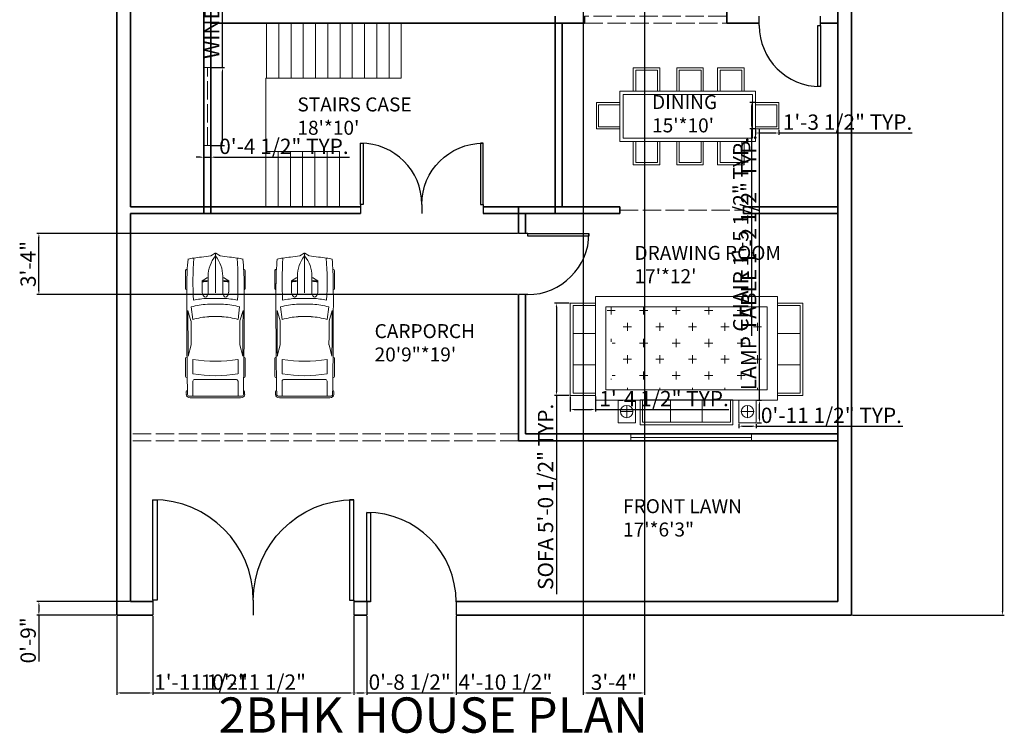
# Model space of a CAD drawing. Units: inches. Extents: x 745 to 1453, y 1850 to 2879.
# Tile 1 of 2: x 745 to 1389, y 1850 to 2316. Entities that reach past the tile are written whole.
import ezdxf

# ---------------------------------------------------------------- set-up
doc = ezdxf.new("R2010")
doc.units = ezdxf.units.IN
doc.linetypes.add('ACAD_ISO02W100', pattern=[15, 12, -3])
for name, color, linetype, lineweight in [('A-ANNO-DIMS', 210, 'Continuous', 18), ('A-ANNO-TEXT', 210, 'Continuous', 25), ('A-AREA-IDEN', 210, 'Continuous', 18), ('A-FLOR-STRS', 92, 'Continuous', 18), ('A-FURN-PATT', 140, 'Continuous', 13), ('A-GLAZ', 4, 'Continuous', 18), ('A-GLAZ-HIGH', 4, 'ACAD_ISO02W100', 18), ('A-WALL-OVHD', 92, 'ACAD_ISO02W100', 18), ('CAR', 10, 'Continuous', 13), ('DOOR', 50, 'Continuous', 25), ('FUR', 140, 'Continuous', 18), ('WALL', 92, 'Continuous', 35)]:
    doc.layers.add(name, color=color, linetype=linetype, lineweight=lineweight)
doc.styles.get("Standard").update_dxf_attribs({"font": 'arial.ttf'})
doc.dimstyles.new('ISO-25', dxfattribs={"dimtxt": 10, "dimasz": 2.5, "dimexe": 1.25, "dimexo": 0.625, "dimtad": 1, "dimdec": 0, "dimlunit": 4, "dimtxsty": 'Standard', "dimcen": 2.5, "dimadec": 0, "dimazin": 0, "dimtfac": 1, "dimtdec": 0, "dimtmove": 0, "dimatfit": 3, "dimfxl": 1, "dimarcsym": 0})

# ---------------------------------------------------------------- blocks, each defined once
blk = doc.blocks.new('*U2')
for p, q in [((0, 0), (0, -6)), ((40, 0), (40, -6))]:
    blk.add_line(p, q)
blk.add_lwpolyline([(0, 0), (0, 40), (1.75, 40), (1.75, 0)], close=True)
blk.add_arc((0, 0), 40, 0, 90)
blk = doc.blocks.new('*U6')
for p, q in [((46.6, 38.9), (22.4, 38.9)), ((136.7, 38.9), (160.9, 38.9)), ((21.1, 37.4), (21.1, 36.8)), ((47.8, 37.4), (47.8, 37.4)), ((70, 31.5), (86.4, 29.4)), ((88, 31.9), (74.8, 35.9)), ((134.3, 35.6), (119.3, 31.8)), ((135.5, 37.1), (135.5, 37.4)), ((138.4, 29.4), (157.2, 29.4)), ((162.1, 37.4), (162.1, 36.8)), ((164.5, 26.4), (164.5, -26.4)), ((186.5, 29.4), (167, 29.4)), ((186.5, -33.5), (186.5, 33.5)), ((188.4, -32.8), (188.4, 32.8)), ((32.3, 11.6), (36.1, 17.2)), ((36.1, 17.2), (50.9, 17.2)), ((3.3, 6.1), (0.1, 0.4)), ((29.8, 9.5), (51.7, 9.5)), ((32.1, 9.5), (32.1, 11.2)), ((58.9, -10.8), (58.9, 10.8)), ((66.6, -10.5), (66.6, 10.5)), ((82.7, 8.5), (82.7, -8.5)), ((186.5, -10.5), (186.5, 10.5)), ((0, 0), (51.7, 0)), ((0.1, -0.4), (3.3, -6.1)), ((29.8, -9.5), (51.7, -9.5)), ((32.1, -9.5), (32.1, -11.2)), ((32.3, -11.6), (36.1, -17.2)), ((36.1, -17.2), (50.9, -17.2)), ((21.1, -37.4), (21.1, -36.8)), ((47.8, -37.4), (47.8, -37.4)), ((86.4, -29.4), (70, -31.5)), ((88, -31.9), (74.8, -35.9)), ((134.3, -35.6), (119.3, -31.8)), ((135.5, -37.1), (135.5, -37.4)), ((157.2, -29.4), (138.4, -29.4)), ((162.1, -37.4), (162.1, -36.8)), ((167, -29.4), (186.5, -29.4)), ((46.6, -38.9), (22.4, -38.9)), ((136.7, -38.9), (160.9, -38.9))]:
    blk.add_line(p, q)
for centre, major_axis, ratio, start_param, end_param in [((22.4, 37.4), (0, -1.48), 0.842304, 3.141593, 4.712389), ((46.6, 37.4), (0, 1.48), 0.842304, -1.570796, 0), ((136.7, 37.4), (0, -1.48), 0.842304, 3.141593, 4.712389), ((160.9, 37.4), (0, 1.48), 0.842304, -1.570796, 0), ((259.2, -27.5), (0, -305.3), 0.842304, 4.528606, 4.561838), ((266, -27.5), (0, 313.3), 0.842304, 1.367076, 1.39176), ((37.5, -594), (0, -623.3), 0.842304, 3.096046, 3.200911), ((41.2, -490.9), (0, 528.2), 0.842304, 0.00281, 0.075598), ((64.5, -10555.6), (0, 10593), 0.842304, -0.013397, 0.002797), ((134.4, 5.4), (0, -89.8), 0.842304, 4.449482, 4.652344), ((135.3, 5.4), (0, 81.8), 0.842304, 1.245306, 1.50788), ((64.5, -10555.6), (0, -10591.5), 0.842304, 3.133765, 3.140441), ((149.6, 2.8), (0, -79.6), 0.842304, 4.372215, 4.640744), ((95.8, -3666.4), (0, -3698.2), 0.842304, 3.134049, 3.144098), ((17.1, 0), (0, 147), 0.842304, 4.511394, 4.913384), ((35.9, 0), (0, 147), 0.842304, 4.511394, 4.913384), ((167, 26.4), (0, 2.96), 0.842304, 0, 1.570796), ((180.6, 35.8), (0, 2.22), 0.842304, -0.013017, 1.249894), ((64.5, -10556.4), (0, 10595.3), 0.842304, -0.013397, -0.013017), ((184, 32.8), (0, -5.25), 0.842304, 1.570796, 3.128196), ((184, 33.5), (0, -2.96), 0.842304, 1.570796, 3.128196), ((-204.5, 52.4), (0, -251), 0.842304, 1.385369, 1.434372), ((13, 17), (0, 27.4), 0.842304, 4.435146, 4.718221), ((14.2, 17), (0, 27.4), 0.842304, 4.435146, 4.718221), ((50.8, 13.3), (6.34, -0.36), 0.603834, -1.395552, 1.581315), ((0.6, 0), (0, -0.74), 0.842304, 4.131459, 5.293319), ((29.8, -46.7), (0, 56.2), 0.842304, 0, 0.590319), ((32.7, 11.2), (0, 0.74), 0.842304, 0.879714, 1.570796), ((-204.5, -52.4), (0, 251), 0.842304, -1.434372, -1.385369), ((29.8, 46.7), (0, 56.2), 0.842304, 2.551274, 3.141593), ((32.7, -11.2), (0, -0.74), 0.842304, 4.712389, 5.403472), ((13, -17), (0, -27.4), 0.842304, 1.564964, 1.848039), ((14.2, -17), (0, -27.4), 0.842304, 1.564964, 1.848039), ((134.4, -5.4), (0, -89.8), 0.842304, -1.510751, -1.307889), ((135.3, -5.4), (0, -81.8), 0.842304, -1.50788, -1.245306), ((149.6, -2.8), (0, -79.6), 0.842304, -1.499151, -1.230623), ((259.2, 27.5), (0, 305.3), 0.842304, 1.721348, 1.754579), ((266, 27.5), (0, 313.3), 0.842304, 1.749832, 1.774517), ((37.5, 594), (0, -623.3), 0.842304, -0.059319, 0.045547), ((41.2, 490.9), (0, -528.2), 0.842304, -0.075598, -0.00281), ((22.4, -37.4), (0, 1.48), 0.842304, 1.570796, 3.141593), ((64.5, 10555.6), (0, 10593), 0.842304, 3.138796, 3.15499), ((46.6, -37.4), (0, -1.48), 0.842304, 0, 1.570796), ((64.5, 10555.6), (0, -10591.5), 0.842304, 0.001152, 0.007828), ((95.8, 3666.4), (0, -3698.2), 0.842304, -0.002505, 0.007544), ((136.7, -37.4), (0, -1.48), 0.842304, -1.570796, 0), ((160.9, -37.4), (0, 1.48), 0.842304, 3.141593, 4.712389), ((167, -26.4), (0, -2.96), 0.842304, 4.712389, 6.283185), ((180.6, -35.8), (0, -2.22), 0.842304, -1.249894, 0.013017), ((64.5, 10556.4), (0, 10595.3), 0.842304, 3.15461, 3.15499), ((184, -32.8), (0, -5.25), 0.842304, 0.013397, 1.570796), ((184, -33.5), (0, 2.96), 0.842304, 3.15499, 4.712389)]:
    blk.add_ellipse(centre, major_axis=major_axis, ratio=ratio, start_param=start_param, end_param=end_param)
at = {"extrusion": (0, 0, -1)}
blk.add_ellipse((50.8, -13.3), major_axis=(6.34, 0.36), ratio=0.603834, start_param=-1.395552, end_param=1.581315, dxfattribs=at)
blk = doc.blocks.new('*D8')
at = {"layer": 'A-ANNO-DIMS', "color": 0, "lineweight": -2, "transparency": 16777216}
for p, q in [((1289.4, 2790.99), (1388.63, 2790.99)), ((1387.38, 2788.49), (1387.38, 1929.49)), ((1289.4, 1926.99), (1388.63, 1926.99))]:
    blk.add_line(p, q, dxfattribs=at)
at = {"layer": 'A-ANNO-DIMS', "color": 0, "lineweight": 100, "transparency": 16777216}
for points in [[(1386.96, 2788.49), (1387.79, 2788.49), (1387.38, 2790.99)], [(1386.96, 1929.49), (1387.79, 1929.49), (1387.38, 1926.99)]]:
    blk.add_solid(points, dxfattribs=at)
at = {"layer": 'Defpoints', "color": 0, "lineweight": 100, "transparency": 16777216}
for p in [(1288.78, 2790.99), (1288.78, 1926.99), (1387.38, 1926.99)]:
    blk.add_point(p, dxfattribs=at)
at = {"layer": 'A-ANNO-DIMS', "color": 0, "transparency": 16777216, "insert": (1381.73, 2358.99), "char_height": 10, "attachment_point": 5, "rotation": 90}
blk.add_mtext("72'", dxfattribs=at)
blk = doc.blocks.new('DINING-CHAIR')
for p, q in [((0, 0), (0, 15.25)), ((0, 15.25), (17.38, 15.25)), ((17.38, 15.25), (17.38, 0)), ((1.66, 0), (0, 0)), ((17.38, 0), (15.91, 0))]:
    blk.add_line(p, q)
blk.add_lwpolyline([(1.66, 0), (15.91, 0), (15.91, 13.88), (1.66, 13.88)], close=True)
blk = doc.blocks.new('LAMP-TABLE-PARLOR')
for p, q in [((9.73, 7.36), (1.61, 7.36)), ((1.61, 7.36), (5.67, 7.36)), ((5.67, 7.36), (5.67, 11.42)), ((5.67, 11.42), (5.67, 3.3)), ((5.67, 7.36), (9.73, 7.36))]:
    blk.add_line(p, q)
blk.add_lwpolyline([(0, 0), (0, 14.73), (11.34, 14.73), (11.34, 0)], close=True)
blk.add_circle((5.67, 7.36), 4.06)
blk = doc.blocks.new('SOFA-3-SEAT')
for p, q in [((1.49, 16.47), (0, 16.47)), ((0, 16.47), (0, 0)), ((19.8, 16.47), (19.8, 1.85)), ((40.42, 16.47), (40.42, 1.85)), ((60.43, 16.47), (58.52, 16.47)), ((60.43, 0), (60.43, 16.47)), ((0, 0), (60.43, 0))]:
    blk.add_line(p, q)
blk.add_lwpolyline([(1.49, 1.85), (1.49, 16.47), (58.88, 16.47), (58.88, 1.85)], close=True)
blk = doc.blocks.new('WINDOW-PASSAGE-51IN')
blk.add_line((2.25, 0), (2.25, 50.89))
blk.add_lwpolyline([(0, 50.89), (4.5, 50.89), (4.5, 0), (0, 0)], close=True)
blk = doc.blocks.new('*D18')
at = {"layer": 'A-ANNO-DIMS', "color": 0, "lineweight": -2, "transparency": 16777216}
for p, q in [((1225.55, 2262.17), (1222.32, 2262.17)), ((1223.57, 2259.67), (1223.57, 2247.29)), ((1225.55, 2244.79), (1222.32, 2244.79)), ((1223.57, 2244.79), (1223.57, 2109.55))]:
    blk.add_line(p, q, dxfattribs=at)
at = {"layer": 'A-ANNO-DIMS', "color": 0, "lineweight": 100, "transparency": 16777216}
for points in [[(1223.15, 2259.67), (1223.99, 2259.67), (1223.57, 2262.17)], [(1223.15, 2247.29), (1223.99, 2247.29), (1223.57, 2244.79)]]:
    blk.add_solid(points, dxfattribs=at)
at = {"layer": 'Defpoints', "color": 0, "lineweight": 100, "transparency": 16777216}
for p in [(1226.18, 2262.17), (1223.57, 2244.79), (1226.18, 2244.79)]:
    blk.add_point(p, dxfattribs=at)
at = {"layer": 'A-ANNO-DIMS', "color": 0, "transparency": 16777216, "insert": (1217.77, 2175.92), "char_height": 10, "attachment_point": 5, "rotation": 90}
blk.add_mtext('CHAIR 1\'-5 1/2" TYP.', dxfattribs=at)
blk = doc.blocks.new('*D19')
at = {"layer": 'A-ANNO-DIMS', "color": 0, "lineweight": -2, "transparency": 16777216}
for p, q in [((1226.18, 2244.17), (1226.18, 2240.93)), ((1228.68, 2242.18), (1238.93, 2242.18)), ((1241.43, 2244.17), (1241.43, 2240.93)), ((1241.43, 2242.18), (1328.5, 2242.18))]:
    blk.add_line(p, q, dxfattribs=at)
at = {"layer": 'A-ANNO-DIMS', "color": 0, "lineweight": 100, "transparency": 16777216}
for points in [[(1228.68, 2242.6), (1228.68, 2241.77), (1226.18, 2242.18)], [(1238.93, 2242.6), (1238.93, 2241.77), (1241.43, 2242.18)]]:
    blk.add_solid(points, dxfattribs=at)
at = {"layer": 'Defpoints', "color": 0, "lineweight": 100, "transparency": 16777216}
for p in [(1226.18, 2244.79), (1241.43, 2244.79), (1241.43, 2242.18)]:
    blk.add_point(p, dxfattribs=at)
at = {"layer": 'A-ANNO-DIMS', "color": 0, "transparency": 16777216, "insert": (1286.21, 2247.98), "char_height": 10, "attachment_point": 5}
blk.add_mtext('1\'-3 1/2" TYP.', dxfattribs=at)
blk = doc.blocks.new('*D30')
at = {"layer": 'A-ANNO-DIMS', "color": 0, "lineweight": -2, "transparency": 16777216}
for p, q in [((1228.75, 2067.48), (1228.75, 2245.1)), ((1227.17, 2067.48), (1230, 2067.48)), ((1228.75, 2055.25), (1228.75, 2064.98)), ((1227.17, 2052.75), (1230, 2052.75))]:
    blk.add_line(p, q, dxfattribs=at)
at = {"layer": 'A-ANNO-DIMS', "color": 0, "lineweight": 100, "transparency": 16777216}
for points in [[(1228.33, 2064.98), (1229.17, 2064.98), (1228.75, 2067.48)], [(1228.33, 2055.25), (1229.17, 2055.25), (1228.75, 2052.75)]]:
    blk.add_solid(points, dxfattribs=at)
at = {"layer": 'Defpoints', "color": 0, "lineweight": 100, "transparency": 16777216}
for p in [(1226.54, 2067.48), (1228.75, 2067.48), (1226.54, 2052.75)]:
    blk.add_point(p, dxfattribs=at)
at = {"layer": 'A-ANNO-DIMS', "color": 0, "transparency": 16777216, "insert": (1222.95, 2157.54), "char_height": 10, "attachment_point": 5, "rotation": 90}
blk.add_mtext('LAMP TABLE 1\'-2 1/2" TYP.', dxfattribs=at)
blk = doc.blocks.new('*D31')
at = {"layer": 'A-ANNO-DIMS', "color": 0, "lineweight": -2, "transparency": 16777216}
for p, q in [((1215.2, 2052.13), (1215.2, 2049.29)), ((1226.54, 2052.13), (1226.54, 2049.29)), ((1217.7, 2050.54), (1224.04, 2050.54)), ((1226.54, 2050.54), (1322.32, 2050.54))]:
    blk.add_line(p, q, dxfattribs=at)
at = {"layer": 'A-ANNO-DIMS', "color": 0, "lineweight": 100, "transparency": 16777216}
for points in [[(1217.7, 2050.96), (1217.7, 2050.13), (1215.2, 2050.54)], [(1224.04, 2050.96), (1224.04, 2050.13), (1226.54, 2050.54)]]:
    blk.add_solid(points, dxfattribs=at)
at = {"layer": 'Defpoints', "color": 0, "lineweight": 100, "transparency": 16777216}
for p in [(1215.2, 2052.75), (1226.54, 2052.75), (1226.54, 2050.54)]:
    blk.add_point(p, dxfattribs=at)
at = {"layer": 'A-ANNO-DIMS', "color": 0, "transparency": 16777216, "insert": (1275.68, 2056.34), "char_height": 10, "attachment_point": 5}
blk.add_mtext('0\'-11 1/2" TYP.', dxfattribs=at)
blk = doc.blocks.new('*D32')
at = {"layer": 'A-ANNO-DIMS', "color": 0, "lineweight": -2, "transparency": 16777216}
for p, q in [((1104.48, 2131), (1094.79, 2131)), ((1096.04, 2128.5), (1096.04, 2073.07)), ((1104.48, 2070.57), (1094.79, 2070.57)), ((1096.04, 2070.57), (1096.04, 1940.69))]:
    blk.add_line(p, q, dxfattribs=at)
at = {"layer": 'A-ANNO-DIMS', "color": 0, "lineweight": 100, "transparency": 16777216}
for points in [[(1095.63, 2128.5), (1096.46, 2128.5), (1096.04, 2131)], [(1095.63, 2073.07), (1096.46, 2073.07), (1096.04, 2070.57)]]:
    blk.add_solid(points, dxfattribs=at)
at = {"layer": 'Defpoints', "color": 0, "lineweight": 100, "transparency": 16777216}
for p in [(1105.11, 2131), (1096.04, 2070.57), (1105.11, 2070.57)]:
    blk.add_point(p, dxfattribs=at)
at = {"layer": 'A-ANNO-DIMS', "color": 0, "transparency": 16777216, "insert": (1090.24, 2004.38), "char_height": 10, "attachment_point": 5, "rotation": 90}
blk.add_mtext('SOFA 5\'-0 1/2" TYP.', dxfattribs=at)
blk = doc.blocks.new('*D33')
at = {"layer": 'A-ANNO-DIMS', "color": 0, "lineweight": -2, "transparency": 16777216}
for p, q in [((1105.11, 2069.94), (1105.11, 2060.25)), ((1121.57, 2069.94), (1121.57, 2060.25)), ((1107.61, 2061.5), (1119.07, 2061.5)), ((1121.57, 2061.5), (1208.64, 2061.5))]:
    blk.add_line(p, q, dxfattribs=at)
at = {"layer": 'A-ANNO-DIMS', "color": 0, "lineweight": 100, "transparency": 16777216}
for points in [[(1107.61, 2061.92), (1107.61, 2061.09), (1105.11, 2061.5)], [(1119.07, 2061.92), (1119.07, 2061.09), (1121.57, 2061.5)]]:
    blk.add_solid(points, dxfattribs=at)
at = {"layer": 'Defpoints', "color": 0, "lineweight": 100, "transparency": 16777216}
for p in [(1105.11, 2070.57), (1121.57, 2070.57), (1121.57, 2061.5)]:
    blk.add_point(p, dxfattribs=at)
at = {"layer": 'A-ANNO-DIMS', "color": 0, "transparency": 16777216, "insert": (1166.36, 2067.3), "char_height": 10, "attachment_point": 5}
blk.add_mtext('1\'-4 1/2" TYP.', dxfattribs=at)
blk = doc.blocks.new('*D34')
at = {"layer": 'A-ANNO-DIMS', "color": 0, "lineweight": -2, "transparency": 16777216}
for p, q in [((877.91, 2284.89), (877.91, 2415.18)), ((870.9, 2284.89), (879.16, 2284.89)), ((877.91, 2236.5), (877.91, 2282.39)), ((870.9, 2234), (879.16, 2234))]:
    blk.add_line(p, q, dxfattribs=at)
at = {"layer": 'A-ANNO-DIMS', "color": 0, "lineweight": 100, "transparency": 16777216}
for points in [[(877.5, 2282.39), (878.33, 2282.39), (877.91, 2284.89)], [(877.5, 2236.5), (878.33, 2236.5), (877.91, 2234)]]:
    blk.add_solid(points, dxfattribs=at)
at = {"layer": 'Defpoints', "color": 0, "lineweight": 100, "transparency": 16777216}
for p in [(870.28, 2284.89), (877.91, 2284.89), (870.28, 2234)]:
    blk.add_point(p, dxfattribs=at)
at = {"layer": 'A-ANNO-DIMS', "color": 0, "transparency": 16777216, "insert": (872.11, 2351.28), "char_height": 10, "attachment_point": 5, "rotation": 90}
blk.add_mtext('WINDOW 4\'-3" TYP.', dxfattribs=at)
blk = doc.blocks.new('*D35')
at = {"layer": 'A-ANNO-DIMS', "color": 0, "lineweight": -2, "transparency": 16777216}
for p, q in [((865.78, 2233.37), (865.78, 2225.12)), ((870.28, 2233.37), (870.28, 2225.12)), ((863.28, 2226.37), (860.78, 2226.37)), ((865.78, 2226.37), (870.28, 2226.37)), ((872.78, 2226.37), (960.79, 2226.37))]:
    blk.add_line(p, q, dxfattribs=at)
at = {"layer": 'A-ANNO-DIMS', "color": 0, "lineweight": 100, "transparency": 16777216}
for points in [[(863.28, 2226.78), (863.28, 2225.95), (865.78, 2226.37)], [(872.78, 2226.78), (872.78, 2225.95), (870.28, 2226.37)]]:
    blk.add_solid(points, dxfattribs=at)
at = {"layer": 'Defpoints', "color": 0, "lineweight": 100, "transparency": 16777216}
for p in [(865.78, 2234), (870.28, 2234), (870.28, 2226.37)]:
    blk.add_point(p, dxfattribs=at)
at = {"layer": 'A-ANNO-DIMS', "color": 0, "transparency": 16777216, "insert": (918.03, 2232.16), "char_height": 10, "attachment_point": 5}
blk.add_mtext('0\'-4 1/2" TYP.', dxfattribs=at)
blk = doc.blocks.new('*D36')
at = {"layer": 'A-ANNO-DIMS', "color": 0, "lineweight": -2, "transparency": 16777216}
for p, q in [((808.78, 1926.36), (808.78, 1874.94)), ((832.39, 1926.36), (832.39, 1874.94)), ((811.28, 1876.19), (829.89, 1876.19)), ((832.39, 1876.19), (892.85, 1876.19))]:
    blk.add_line(p, q, dxfattribs=at)
at = {"layer": 'A-ANNO-DIMS', "color": 0, "lineweight": 100, "transparency": 16777216}
for points in [[(811.28, 1876.6), (811.28, 1875.77), (808.78, 1876.19)], [(829.89, 1876.6), (829.89, 1875.77), (832.39, 1876.19)]]:
    blk.add_solid(points, dxfattribs=at)
at = {"layer": 'Defpoints', "color": 0, "lineweight": 100, "transparency": 16777216}
for p in [(808.78, 1926.99), (832.39, 1926.99), (832.39, 1876.19)]:
    blk.add_point(p, dxfattribs=at)
at = {"layer": 'A-ANNO-DIMS', "color": 0, "transparency": 16777216, "insert": (863.87, 1881.98), "char_height": 10, "attachment_point": 5}
blk.add_mtext('1\'-11 1/2"', dxfattribs=at)
blk = doc.blocks.new('*D37')
at = {"layer": 'A-ANNO-DIMS', "color": 0, "lineweight": -2, "transparency": 16777216}
for p, q in [((832.39, 1926.36), (832.39, 1874.94)), ((963.67, 1926.36), (963.67, 1874.94)), ((834.89, 1876.19), (961.17, 1876.19))]:
    blk.add_line(p, q, dxfattribs=at)
at = {"layer": 'A-ANNO-DIMS', "color": 0, "lineweight": 100, "transparency": 16777216}
for points in [[(834.89, 1876.6), (834.89, 1875.77), (832.39, 1876.19)], [(961.17, 1876.6), (961.17, 1875.77), (963.67, 1876.19)]]:
    blk.add_solid(points, dxfattribs=at)
at = {"layer": 'Defpoints', "color": 0, "lineweight": 100, "transparency": 16777216}
for p in [(832.39, 1926.99), (963.67, 1926.99), (963.67, 1876.19)]:
    blk.add_point(p, dxfattribs=at)
at = {"layer": 'A-ANNO-DIMS', "color": 0, "transparency": 16777216, "insert": (898.03, 1881.98), "char_height": 10, "attachment_point": 5}
blk.add_mtext('10\'-11 1/2"', dxfattribs=at)
blk = doc.blocks.new('*D38')
at = {"layer": 'A-ANNO-DIMS', "color": 0, "lineweight": -2, "transparency": 16777216}
for p, q in [((963.67, 1926.36), (963.67, 1874.94)), ((972.12, 1926.36), (972.12, 1874.94)), ((966.17, 1876.19), (969.62, 1876.19)), ((972.12, 1876.19), (1025.75, 1876.19))]:
    blk.add_line(p, q, dxfattribs=at)
at = {"layer": 'A-ANNO-DIMS', "color": 0, "lineweight": 100, "transparency": 16777216}
for points in [[(966.17, 1876.6), (966.17, 1875.77), (963.67, 1876.19)], [(969.62, 1876.6), (969.62, 1875.77), (972.12, 1876.19)]]:
    blk.add_solid(points, dxfattribs=at)
at = {"layer": 'Defpoints', "color": 0, "lineweight": 100, "transparency": 16777216}
for p in [(963.67, 1926.99), (972.12, 1926.99), (972.12, 1876.19)]:
    blk.add_point(p, dxfattribs=at)
at = {"layer": 'A-ANNO-DIMS', "color": 0, "transparency": 16777216, "insert": (1000.18, 1881.98), "char_height": 10, "attachment_point": 5}
blk.add_mtext('0\'-8 1/2"', dxfattribs=at)
blk = doc.blocks.new('*D39')
at = {"layer": 'A-ANNO-DIMS', "color": 0, "lineweight": -2, "transparency": 16777216}
for p, q in [((972.12, 1926.36), (972.12, 1874.94)), ((1030.53, 1926.36), (1030.53, 1874.94)), ((974.62, 1876.19), (1028.03, 1876.19)), ((1030.53, 1876.19), (1092.34, 1876.19))]:
    blk.add_line(p, q, dxfattribs=at)
at = {"layer": 'A-ANNO-DIMS', "color": 0, "lineweight": 100, "transparency": 16777216}
for points in [[(974.62, 1876.6), (974.62, 1875.77), (972.12, 1876.19)], [(1028.03, 1876.6), (1028.03, 1875.77), (1030.53, 1876.19)]]:
    blk.add_solid(points, dxfattribs=at)
at = {"layer": 'Defpoints', "color": 0, "lineweight": 100, "transparency": 16777216}
for p in [(972.12, 1926.99), (1030.53, 1926.99), (1030.53, 1876.19)]:
    blk.add_point(p, dxfattribs=at)
at = {"layer": 'A-ANNO-DIMS', "color": 0, "transparency": 16777216, "insert": (1062.69, 1881.98), "char_height": 10, "attachment_point": 5}
blk.add_mtext('4\'-10 1/2"', dxfattribs=at)
blk = doc.blocks.new('*D40')
at = {"layer": 'A-ANNO-DIMS', "color": 0, "lineweight": -2, "transparency": 16777216}
for p, q in [((817.15, 1935.99), (756.73, 1935.99)), ((757.98, 1933.49), (757.98, 1929.49)), ((808.15, 1926.99), (756.73, 1926.99)), ((757.98, 1926.99), (757.98, 1896.65))]:
    blk.add_line(p, q, dxfattribs=at)
at = {"layer": 'A-ANNO-DIMS', "color": 0, "lineweight": 100, "transparency": 16777216}
for points in [[(757.56, 1933.49), (758.4, 1933.49), (757.98, 1935.99)], [(757.56, 1929.49), (758.4, 1929.49), (757.98, 1926.99)]]:
    blk.add_solid(points, dxfattribs=at)
at = {"layer": 'Defpoints', "color": 0, "lineweight": 100, "transparency": 16777216}
for p in [(817.78, 1935.99), (757.98, 1926.99), (808.78, 1926.99)]:
    blk.add_point(p, dxfattribs=at)
at = {"layer": 'A-ANNO-DIMS', "color": 0, "transparency": 16777216, "insert": (752.25, 1910.57), "char_height": 10, "attachment_point": 5, "rotation": 90}
blk.add_mtext('0\'-9"', dxfattribs=at)
blk = doc.blocks.new('*D41')
at = {"layer": 'A-ANNO-DIMS', "color": 0, "lineweight": -2, "transparency": 16777216}
for p, q in [((1113.55, 2526.36), (1113.55, 1874.94)), ((1153.55, 2526.36), (1153.55, 1874.94)), ((1116.05, 1876.19), (1151.05, 1876.19))]:
    blk.add_line(p, q, dxfattribs=at)
at = {"layer": 'A-ANNO-DIMS', "color": 0, "lineweight": 100, "transparency": 16777216}
for points in [[(1116.05, 1876.6), (1116.05, 1875.77), (1113.55, 1876.19)], [(1151.05, 1876.6), (1151.05, 1875.77), (1153.55, 1876.19)]]:
    blk.add_solid(points, dxfattribs=at)
at = {"layer": 'Defpoints', "color": 0, "lineweight": 100, "transparency": 16777216}
for p in [(1113.55, 2526.99), (1153.55, 2526.99), (1153.55, 1876.19)]:
    blk.add_point(p, dxfattribs=at)
at = {"layer": 'A-ANNO-DIMS', "color": 0, "transparency": 16777216, "insert": (1133.55, 1881.92), "char_height": 10, "attachment_point": 5}
blk.add_mtext('3\'-4"', dxfattribs=at)
blk = doc.blocks.new('*D42')
at = {"layer": 'A-ANNO-DIMS', "color": 0, "lineweight": -2, "transparency": 16777216}
for p, q in [((1070.65, 2176.56), (756.73, 2176.56)), ((757.98, 2139.06), (757.98, 2174.06)), ((1070.65, 2136.56), (756.73, 2136.56))]:
    blk.add_line(p, q, dxfattribs=at)
at = {"layer": 'A-ANNO-DIMS', "color": 0, "lineweight": 100, "transparency": 16777216}
for points in [[(757.56, 2174.06), (758.4, 2174.06), (757.98, 2176.56)], [(757.56, 2139.06), (758.4, 2139.06), (757.98, 2136.56)]]:
    blk.add_solid(points, dxfattribs=at)
at = {"layer": 'Defpoints', "color": 0, "lineweight": 100, "transparency": 16777216}
for p in [(757.98, 2176.56), (1071.28, 2176.56), (1071.28, 2136.56)]:
    blk.add_point(p, dxfattribs=at)
at = {"layer": 'A-ANNO-DIMS', "color": 0, "transparency": 16777216, "insert": (752.24, 2156.56), "char_height": 10, "attachment_point": 5, "rotation": 90}
blk.add_mtext('3\'-4"', dxfattribs=at)

msp = doc.modelspace()

# ---------------------------------------------------------------- hatches: boundary and pattern name
at = {"layer": 'A-FURN-PATT'}
h = msp.add_hatch(dxfattribs=at)
h.set_pattern_fill('CROSS', color=256, scale=1.673314, angle=-90)
h.set_pattern_definition([(270, (-3129.103, 4179.532), (10.625542, -10.625542), [5.31277, -15.938313]), (360, (-3131.759, 4176.875), (10.625542, 10.625542), [5.31277, -15.938313])])
h.paths.add_polyline_path([(1128.38, 2128.49), (1128.38, 2105.7), (1132.49, 2105.7), (1132.49, 2103.98), (1132.49, 2083.25), (1132.49, 2081.49), (1128.38, 2081.49), (1128.38, 2074.28), (1233.7, 2074.28), (1233.7, 2128.49)])

# ---------------------------------------------------------------- linework, layer by layer
at = {"layer": 'A-FLOR-STRS'}
for p, q in [((870.28, 2313.99), (906.28, 2313.99)), ((906.69, 2313.99), (906.69, 2277.99)), ((914.69, 2313.99), (914.69, 2277.99)), ((922.69, 2313.99), (922.69, 2277.99)), ((930.69, 2313.99), (930.69, 2277.99)), ((938.69, 2313.99), (938.69, 2277.99)), ((946.69, 2313.99), (946.69, 2277.99)), ((954.69, 2313.99), (954.69, 2277.99)), ((962.69, 2313.99), (962.69, 2277.99)), ((970.69, 2313.99), (970.69, 2277.99)), ((978.69, 2313.99), (978.69, 2277.99)), ((986.69, 2313.99), (986.69, 2277.99)), ((994.69, 2313.99), (994.69, 2277.99)), ((994.69, 2277.99), (906.28, 2277.99)), ((906.28, 2277.99), (906.28, 2229.99)), ((870.28, 2193.99), (870.28, 2229.99)), ((906.28, 2229.99), (938.25, 2229.99)), ((906.28, 2229.99), (906.28, 2193.99)), ((914.28, 2229.99), (914.28, 2193.99)), ((922.28, 2229.99), (922.28, 2193.99)), ((930.28, 2229.99), (930.28, 2193.99)), ((938.28, 2229.99), (938.28, 2193.99)), ((938.28, 2229.99), (954.28, 2229.99)), ((946.28, 2229.99), (946.28, 2193.99)), ((954.28, 2229.99), (954.28, 2193.99))]:
    msp.add_line(p, q, dxfattribs=at)
at = {"layer": 'A-GLAZ'}
msp.add_line((1144.55, 2043.24), (1223.57, 2043.24), dxfattribs=at)
msp.add_lwpolyline([(1144.55, 2045.49), (1223.57, 2045.49), (1223.57, 2040.99), (1144.55, 2040.99)], close=True, dxfattribs=at)
at = {"layer": 'A-WALL-OVHD'}
for p, q in [((1137.41, 2191.74), (1218.36, 2191.74)), ((1071.28, 2045.49), (817.78, 2045.49)), ((1071.28, 2040.99), (817.78, 2040.99))]:
    msp.add_line(p, q, dxfattribs=at)
msp.add_lwpolyline([(1207.28, 2318.49), (1114.37, 2318.49), (1114.37, 2313.99), (1207.28, 2313.99)], close=True, dxfattribs=at)
at = {"layer": 'FUR'}
for p, q in [((1240.56, 2131), (1257.03, 2131)), ((1257.03, 2131), (1257.03, 2070.57)), ((1240.56, 2111.2), (1255.18, 2111.2)), ((1121.57, 2083.25), (1121.57, 2103.98)), ((1128.38, 2083.25), (1128.38, 2103.98)), ((1240.56, 2090.58), (1255.18, 2090.58)), ((1257.03, 2070.57), (1240.56, 2070.57))]:
    msp.add_line(p, q, dxfattribs=at)
for points in [[(1137.45, 2269.45), (1226.18, 2269.45), (1226.18, 2236.72), (1137.45, 2236.72)], [(1139.57, 2267.34), (1224.06, 2267.34), (1224.06, 2238.83), (1139.57, 2238.83)], [(1255.18, 2129.51), (1240.56, 2129.51), (1240.56, 2072.12), (1255.18, 2072.12)]]:
    msp.add_lwpolyline(points, close=True, dxfattribs=at)
for points in [[(1121.57, 2083.25), (1121.57, 2067.48), (1240.51, 2067.48), (1240.51, 2135.3), (1121.57, 2135.3), (1121.57, 2103.98)], [(1128.38, 2083.25), (1128.38, 2074.28), (1233.7, 2074.28), (1233.7, 2128.49), (1128.38, 2128.49), (1128.38, 2103.98)]]:
    msp.add_lwpolyline(points, dxfattribs=at)
at = {"layer": 'WALL'}
for p, q in [((808.78, 1926.99), (808.78, 2790.99)), ((1288.78, 2790.99), (1288.78, 1926.99)), ((817.78, 2193.99), (817.78, 2781.99)), ((1279.78, 2781.99), (1279.78, 1935.99)), ((865.78, 2453.25), (865.78, 2189.49)), ((870.28, 2453.25), (870.28, 2189.49)), ((1207.28, 2313.99), (1207.28, 2420.49)), ((1095.28, 2318.49), (1095.28, 2189.49)), ((1114.37, 2313.99), (1114.37, 2318.49)), ((870.28, 2189.49), (870.28, 2313.99)), ((870.28, 2313.99), (1086.28, 2313.99)), ((1086.28, 2313.99), (1106.47, 2313.99)), ((1099.78, 2313.99), (1099.78, 2193.99)), ((1114.37, 2313.99), (1099.78, 2313.99)), ((1228.51, 2313.99), (1207.28, 2313.99)), ((1228.51, 2313.99), (1207.28, 2313.99)), ((1279.78, 2313.99), (1268.51, 2313.99)), ((1279.78, 2313.99), (1268.51, 2313.99)), ((968.14, 2193.99), (817.78, 2193.99)), ((1071.28, 2193.99), (1048.14, 2193.99)), ((1071.28, 2193.99), (1071.28, 2176.56)), ((1137.41, 2193.99), (1071.28, 2193.99)), ((1099.78, 2193.99), (1137.41, 2193.99)), ((1137.41, 2189.49), (1137.41, 2193.99)), ((1279.78, 2193.99), (1218.36, 2193.99)), ((1218.36, 2189.49), (1218.36, 2193.99)), ((1218.36, 2193.99), (1279.78, 2193.99)), ((817.78, 1935.99), (817.78, 2189.49)), ((968.14, 2189.49), (817.78, 2189.49)), ((1080, 2189.49), (1048.14, 2189.49)), ((1075.78, 2189.49), (1075.78, 2176.56)), ((1137.41, 2189.49), (1075.78, 2189.49)), ((1095.28, 2189.49), (1137.41, 2189.49)), ((1279.78, 2189.49), (1218.36, 2189.49)), ((1218.36, 2189.49), (1279.78, 2189.49)), ((1071.28, 2136.56), (1071.28, 2040.99)), ((1075.78, 2136.56), (1075.78, 2045.49)), ((1075.78, 2045.49), (1279.78, 2045.49)), ((1071.28, 2040.99), (1279.78, 2040.99)), ((832.39, 1935.99), (817.78, 1935.99)), ((974.67, 1935.99), (963.67, 1935.99)), ((1279.78, 1935.99), (1030.53, 1935.99)), ((832.39, 1926.99), (808.78, 1926.99)), ((972.12, 1926.99), (963.67, 1926.99)), ((1288.78, 1926.99), (1030.53, 1926.99))]:
    msp.add_line(p, q, dxfattribs=at)

# ---------------------------------------------------------------- block references
at = {"layer": 'A-GLAZ-HIGH'}
msp.add_blockref('WINDOW-PASSAGE-51IN', (865.78, 2234), dxfattribs=at)
at = {"layer": 'CAR', "xscale": 0.5012918227692138, "yscale": 0.5012918227692138, "zscale": 0.5012918227692138, "rotation": 270}
for p in [(873.32, 2163.59), (931.57, 2163.59)]:
    msp.add_blockref('*U6', p, dxfattribs=at)
at = {"layer": 'DOOR'}
for p, rotation in [((1268.51, 2312.49), 180), ((1077.28, 2176.56), 270)]:
    msp.add_blockref('*U2', p, dxfattribs=dict(at, rotation=rotation))
msp.add_blockref('*U2', (968.14, 2195.49), dxfattribs=at)
at = {"layer": 'DOOR', "xscale": -1}
msp.add_blockref('*U2', (1048.14, 2195.49), dxfattribs=at)
at = {"layer": 'DOOR'}
for p, xscale, yscale, zscale in [((832.39, 1936.83), 1.64100367937049, 1.64100367937049, 1.64100367937049), ((963.67, 1936.83), -1.64100367937049, 1.64100367937049, 1.64100367937049), ((972.12, 1935.75), 1.460450166984614, 1.460450166984614, 1.460450166984614)]:
    msp.add_blockref('*U2', p, dxfattribs=dict(at, xscale=xscale, yscale=yscale, zscale=zscale))
at = {"layer": 'FUR'}
for name, p in [('DINING-CHAIR', (1146.2, 2269.45)), ('DINING-CHAIR', (1174.61, 2269.45)), ('DINING-CHAIR', (1201.3, 2269.45)), ('LAMP-TABLE-PARLOR', (1136.29, 2052.75)), ('SOFA-3-SEAT', (1150.84, 2051.4)), ('LAMP-TABLE-PARLOR', (1215.2, 2052.75))]:
    msp.add_blockref(name, p, dxfattribs=at)
at = {"layer": 'FUR', "extrusion": (0, 0, -1), "zscale": -1}
for p, rotation in [((-1137.45, 2262.17), 269.9999999999986), ((-1146.2, 2236.72), 180), ((-1174.61, 2236.72), 180), ((-1201.3, 2236.72), 180)]:
    msp.add_blockref('DINING-CHAIR', p, dxfattribs=dict(at, rotation=rotation))
at = {"layer": 'FUR'}
for name, p, rotation in [('DINING-CHAIR', (1226.18, 2262.17), 269.9999999999986), ('SOFA-3-SEAT', (1105.11, 2131), 270.0000000000011)]:
    msp.add_blockref(name, p, dxfattribs=dict(at, rotation=rotation))

# ---------------------------------------------------------------- texts
at = {"layer": 'A-ANNO-TEXT', "insert": (875.4, 1873.27), "char_height": 23.0467, "attachment_point": 1}
msp.add_mtext_dynamic_manual_height_columns('2BHK HOUSE PLAN', width=3350.5382, gutter_width=115.23, heights=[0], dxfattribs=at)
at = {"layer": 'A-AREA-IDEN', "attachment_point": 1}
for s, insert, char_height in [("STAIRS CASE\\P18'*10'", (926.85, 2265.41), 9.1453), ("DINING\\P15'*10'", (1158.53, 2266.98), 9.145), ("DRAWING ROOM\\P17'*12'", (1147.05, 2168.39), 9.1453), ('CARPORCH\\P20\'9"*19\'', (977.26, 2117.25), 9.145), ('FRONT LAWN\\P17\'*6\'3"', (1139.59, 2002.84), 9.145)]:
    msp.add_mtext_dynamic_manual_height_columns(s, width=282.6971, gutter_width=45.73, heights=[0], dxfattribs=dict(at, insert=insert, char_height=char_height))

# ---------------------------------------------------------------- dimensions: what is measured, and where the dimension line sits
at = {"layer": 'A-ANNO-DIMS'}
for base, p1, p2, override, picture, middle in [((1387.38, 1926.99), (1288.78, 2790.99), (1288.78, 1926.99), {"dimclrd": 0, "dimclre": 0, "dimclrt": 0}, '*D8', (1381.73, 2358.99)), ((757.98, 2176.56), (1071.28, 2136.56), (1071.28, 2176.56), {"dimdec": 1, "dimlfac": 1, "dimrnd": 0, "dimzin": 1, "dimdsep": 46, "dimlunit": 4, "dimfrac": 2}, '*D42', (752.24, 2156.56)), ((757.98, 1926.99), (817.78, 1935.99), (808.78, 1926.99), {"dimdec": 1, "dimlfac": 1, "dimrnd": 0, "dimzin": 1, "dimdsep": 46, "dimlunit": 4, "dimfrac": 2}, '*D40', (752.25, 1910.57))]:
    dim = msp.add_linear_dim(base=base, p1=p1, p2=p2, angle=90, dimstyle='ISO-25', override=override, dxfattribs=at)
    dim.commit()
    dim.dimension.update_dxf_attribs({"geometry": picture, "text_midpoint": middle})
for base, p1, p2, picture, middle in [((1153.55, 1876.19), (1113.55, 2526.99), (1153.55, 2526.99), '*D41', (1133.55, 1881.92)), ((832.39, 1876.19), (808.78, 1926.99), (832.39, 1926.99), '*D36', (863.87, 1881.98)), ((963.67, 1876.19), (832.39, 1926.99), (963.67, 1926.99), '*D37', (898.03, 1881.98)), ((972.1166, 1876.1867), (963.6688, 1926.9867), (972.1166, 1926.9867), '*D38', (1000.1836, 1881.9822)), ((1030.53, 1876.19), (972.12, 1926.99), (1030.53, 1926.99), '*D39', (1062.69, 1881.98))]:
    dim = msp.add_linear_dim(base=base, p1=p1, p2=p2, dimstyle='ISO-25', override={"dimdec": 1, "dimlfac": 1, "dimrnd": 0, "dimzin": 1, "dimdsep": 46, "dimlunit": 4, "dimfrac": 2}, dxfattribs=at)
    dim.commit()
    dim.dimension.update_dxf_attribs({"geometry": picture, "text_midpoint": middle})
for base, p1, p2, angle, text, picture, middle in [((877.91, 2284.89), (870.28, 2234), (870.28, 2284.89), 90, 'WINDOW <> TYP.', '*D34', (872.11, 2351.28)), ((1223.57, 2244.79), (1226.18, 2262.17), (1226.18, 2244.79), 270, 'CHAIR <> TYP.', '*D18', (1217.77, 2175.92)), ((1228.75, 2067.48), (1226.54, 2052.75), (1226.54, 2067.48), 90, 'LAMP TABLE <> TYP.', '*D30', (1222.95, 2157.54)), ((1096.04, 2070.57), (1105.11, 2131), (1105.11, 2070.57), 270, 'SOFA <> TYP.', '*D32', (1090.24, 2004.38)), ((1121.57, 2061.5), (1105.11, 2070.57), (1121.57, 2070.57), 0, '<> TYP.', '*D33', (1166.36, 2067.3))]:
    dim = msp.add_linear_dim(base=base, p1=p1, p2=p2, angle=angle, text=text, dimstyle='ISO-25', override={"dimdec": 1, "dimlfac": 1, "dimrnd": 0, "dimzin": 1, "dimdsep": 46, "dimlunit": 4, "dimfrac": 2}, dxfattribs=at)
    dim.commit()
    dim.dimension.update_dxf_attribs({"geometry": picture, "text_midpoint": middle})
for base, p1, p2, picture, middle in [((1241.4309, 2242.1828), (1226.1764, 2244.7902), (1241.4309, 2244.7902), '*D19', (1286.2134, 2247.9817)), ((870.28, 2226.37), (865.78, 2234), (870.28, 2234), '*D35', (918.03, 2232.16)), ((1226.54, 2050.54), (1215.2, 2052.75), (1226.54, 2052.75), '*D31', (1275.68, 2056.34))]:
    dim = msp.add_linear_dim(base=base, p1=p1, p2=p2, text='<> TYP.', dimstyle='ISO-25', override={"dimdec": 1, "dimlfac": 1, "dimrnd": 0, "dimzin": 1, "dimdsep": 46, "dimlunit": 4, "dimfrac": 2}, dxfattribs=at)
    dim.commit()
    dim.dimension.update_dxf_attribs({"geometry": picture, "text_midpoint": middle})

doc.saveas('drawing.dxf')
